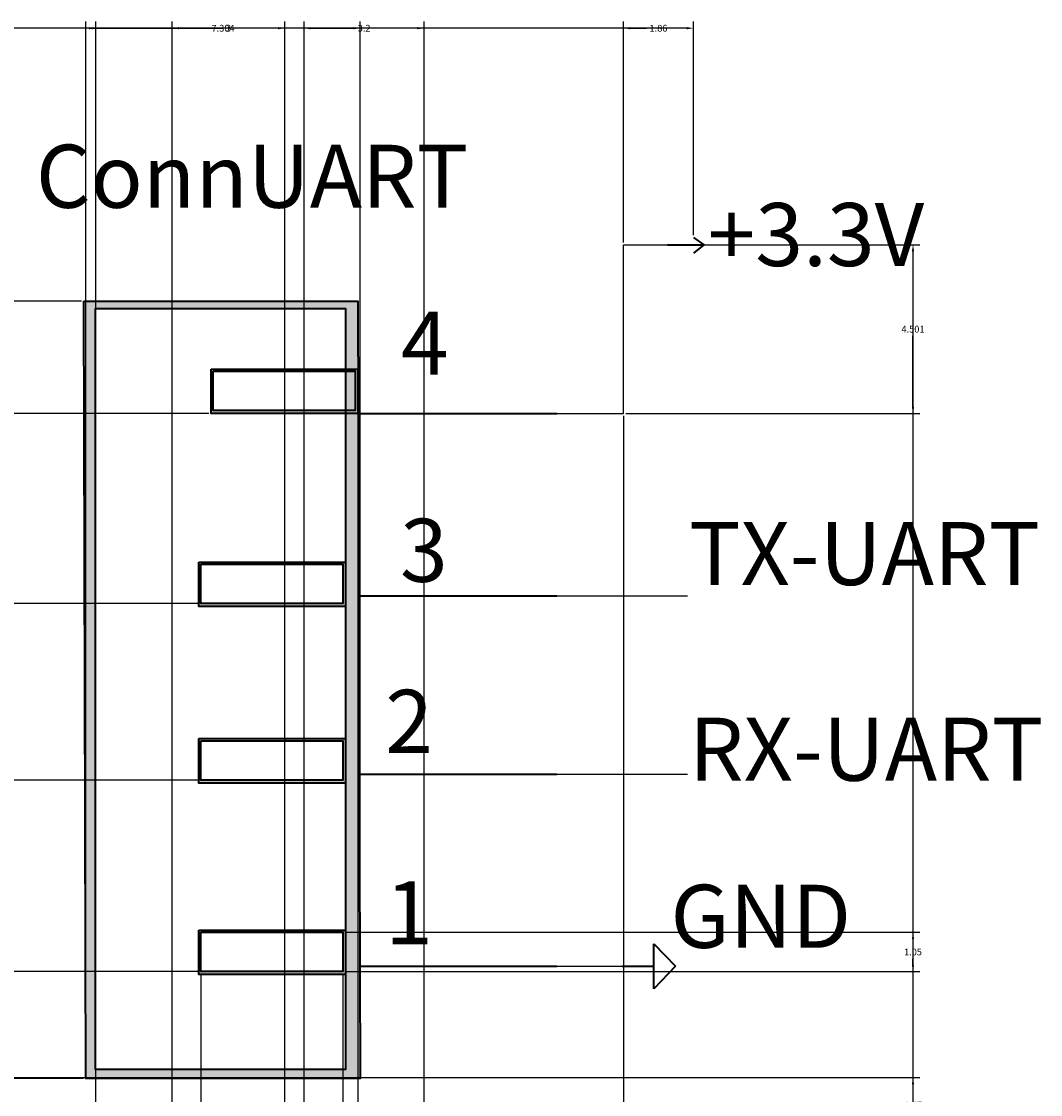
# Model space of a CAD drawing. Units: inches. Extents: x 23 to 132, y 5 to 105.
# Tile 14 of 14: x 105 to 132, y 77 to 105. Entities that reach past the tile are written whole.
import ezdxf

# ---------------------------------------------------------------- set-up
doc = ezdxf.new("R2010")
doc.units = ezdxf.units.IN
doc.header["$MEASUREMENT"] = 0
for name, color, linetype, lineweight in [('A-ANNO-DIMS', 2, 'Continuous', 18), ('E-ANNO-IDEN', 4, 'Continuous', 18), ('E-ANNO-TEXT', 3, 'Continuous', 18), ('E-SYMB', 1, 'Continuous', 35), ('E-SYMB-PATT', 1, 'Continuous', 18), ('E-WIRE', 3, 'Continuous', 25)]:
    doc.layers.add(name, color=color, linetype=linetype, lineweight=lineweight)
doc.styles.get("Standard").update_dxf_attribs({"font": 'arial.ttf'})
doc.dimstyles.get("Standard").update_dxf_attribs({"dimtxt": 0.18, "dimasz": 0.18, "dimexe": 0.18, "dimexo": 0.0625, "dimgap": 0.09, "dimtad": 0, "dimtih": 1, "dimtoh": 1, "dimdec": 4, "dimzin": 0, "dimdsep": 46, "dimtxsty": 'Standard', "dimcen": 0.09, "dimadec": 0, "dimazin": 0, "dimtfac": 1, "dimtdec": 4, "dimtofl": 0, "dimtmove": 0, "dimatfit": 3, "dimfxl": 1, "dimtolj": 1, "dimtzin": 0, "dimarcsym": 0})

# ---------------------------------------------------------------- blocks, each defined once
blk = doc.blocks.new('*D2')
at = {"layer": 'A-ANNO-DIMS', "color": 0, "lineweight": -2, "transparency": 16777216}
for p, q in [((28.697, 66.272), (28.697, 105.232)), ((123.211, 99.539), (123.211, 105.232)), ((28.877, 105.052), (75.577, 105.052)), ((123.031, 105.052), (76.33, 105.052))]:
    blk.add_line(p, q, dxfattribs=at)
at = {"layer": 'A-ANNO-DIMS', "color": 0, "transparency": 16777216}
for points in [[(28.877, 105.082), (28.877, 105.022), (28.697, 105.052)], [(123.031, 105.082), (123.031, 105.022), (123.211, 105.052)]]:
    blk.add_solid(points, dxfattribs=at)
at = {"layer": 'Defpoints', "color": 0, "transparency": 16777216}
for p in [(123.211, 105.052), (123.211, 99.477), (28.697, 66.21)]:
    blk.add_point(p, dxfattribs=at)
at = {"layer": 'A-ANNO-DIMS', "color": 0, "transparency": 16777216, "insert": (75.954, 105.052), "char_height": 0.18, "attachment_point": 5}
blk.add_mtext('\\A1;94.51', dxfattribs=at)
blk = doc.blocks.new('*D3')
at = {"layer": 'A-ANNO-DIMS', "color": 0, "lineweight": -2, "transparency": 16777216}
for p, q in [((121.409, 99.285), (129.239, 99.285)), ((129.059, 99.105), (129.059, 55.423)), ((129.059, 11.378), (129.059, 55.06)), ((72.981, 11.198), (129.239, 11.198))]:
    blk.add_line(p, q, dxfattribs=at)
at = {"layer": 'A-ANNO-DIMS', "color": 0, "transparency": 16777216}
for points in [[(129.029, 99.105), (129.089, 99.105), (129.059, 99.285)], [(129.029, 11.378), (129.089, 11.378), (129.059, 11.198)]]:
    blk.add_solid(points, dxfattribs=at)
at = {"layer": 'Defpoints', "color": 0, "transparency": 16777216}
for p in [(121.346, 99.285), (129.059, 99.285), (72.919, 11.198)]:
    blk.add_point(p, dxfattribs=at)
at = {"layer": 'A-ANNO-DIMS', "color": 0, "transparency": 16777216, "insert": (129.059, 55.241), "char_height": 0.18, "attachment_point": 5}
blk.add_mtext('\\A1;88.09', dxfattribs=at)
blk = doc.blocks.new('*D15')
at = {"layer": 'A-ANNO-DIMS', "color": 0, "lineweight": -2, "transparency": 16777216}
for p, q in [((50.327, 77.095), (129.239, 77.095)), ((129.059, 76.915), (129.059, 76.538)), ((129.059, 75.801), (129.059, 76.177)), ((47.783, 75.621), (129.239, 75.621))]:
    blk.add_line(p, q, dxfattribs=at)
at = {"layer": 'A-ANNO-DIMS', "color": 0, "transparency": 16777216}
for points in [[(129.029, 76.915), (129.089, 76.915), (129.059, 77.095)], [(129.029, 75.801), (129.089, 75.801), (129.059, 75.621)]]:
    blk.add_solid(points, dxfattribs=at)
at = {"layer": 'Defpoints', "color": 0, "transparency": 16777216}
for p in [(50.265, 77.095), (47.72, 75.621), (129.059, 75.621)]:
    blk.add_point(p, dxfattribs=at)
at = {"layer": 'A-ANNO-DIMS', "color": 0, "transparency": 16777216, "insert": (129.059, 76.358), "char_height": 0.18, "attachment_point": 5}
blk.add_mtext('\\A1;1.47', dxfattribs=at)
blk = doc.blocks.new('*D24')
at = {"layer": 'A-ANNO-DIMS', "color": 0, "lineweight": -2, "transparency": 16777216}
for p, q in [((81.032, 77.095), (129.239, 77.095)), ((129.059, 76.915), (129.059, 76.509)), ((129.059, 75.739), (129.059, 76.145)), ((83.576, 75.559), (129.239, 75.559))]:
    blk.add_line(p, q, dxfattribs=at)
at = {"layer": 'A-ANNO-DIMS', "color": 0, "transparency": 16777216}
for points in [[(129.029, 76.915), (129.089, 76.915), (129.059, 77.095)], [(129.029, 75.739), (129.089, 75.739), (129.059, 75.559)]]:
    blk.add_solid(points, dxfattribs=at)
at = {"layer": 'Defpoints', "color": 0, "transparency": 16777216}
for p in [(80.969, 77.095), (83.514, 75.559), (129.059, 75.559)]:
    blk.add_point(p, dxfattribs=at)
at = {"layer": 'A-ANNO-DIMS', "color": 0, "transparency": 16777216, "insert": (129.059, 76.327), "char_height": 0.18, "attachment_point": 5}
blk.add_mtext('\\A1;1.54', dxfattribs=at)
blk = doc.blocks.new('*D49')
at = {"layer": 'A-ANNO-DIMS', "color": 0, "lineweight": -2, "transparency": 16777216}
for p, q in [((83.514, 75.622), (83.514, 105.232)), ((107.287, 75.622), (107.287, 105.232)), ((83.694, 105.052), (94.936, 105.052)), ((107.107, 105.052), (95.865, 105.052))]:
    blk.add_line(p, q, dxfattribs=at)
at = {"layer": 'A-ANNO-DIMS', "color": 0, "transparency": 16777216}
for points in [[(83.694, 105.082), (83.694, 105.022), (83.514, 105.052)], [(107.107, 105.082), (107.107, 105.022), (107.287, 105.052)]]:
    blk.add_solid(points, dxfattribs=at)
at = {"layer": 'Defpoints', "color": 0, "transparency": 16777216}
for p in [(107.287, 105.052), (83.514, 75.559), (107.287, 75.559)]:
    blk.add_point(p, dxfattribs=at)
at = {"layer": 'A-ANNO-DIMS', "color": 0, "transparency": 16777216, "insert": (95.4, 105.052), "char_height": 0.18, "attachment_point": 5}
blk.add_mtext('\\A1;23.774', dxfattribs=at)
blk = doc.blocks.new('*D77')
at = {"layer": 'A-ANNO-DIMS', "color": 0, "lineweight": -2, "transparency": 16777216}
for p, q in [((112.835, 67.751), (112.835, 105.232)), ((116.035, 67.751), (116.035, 105.232)), ((113.015, 105.052), (114.182, 105.052)), ((115.855, 105.052), (114.688, 105.052))]:
    blk.add_line(p, q, dxfattribs=at)
at = {"layer": 'A-ANNO-DIMS', "color": 0, "transparency": 16777216}
for points in [[(113.015, 105.082), (113.015, 105.022), (112.835, 105.052)], [(115.855, 105.082), (115.855, 105.022), (116.035, 105.052)]]:
    blk.add_solid(points, dxfattribs=at)
at = {"layer": 'Defpoints', "color": 0, "transparency": 16777216}
for p in [(116.035, 105.052), (112.835, 67.688), (116.035, 67.688)]:
    blk.add_point(p, dxfattribs=at)
at = {"layer": 'A-ANNO-DIMS', "color": 0, "transparency": 16777216, "insert": (114.435, 105.052), "char_height": 0.18, "attachment_point": 5}
blk.add_mtext('\\A1;3.2', dxfattribs=at)
blk = doc.blocks.new('*D82')
at = {"layer": 'A-ANNO-DIMS', "color": 0, "lineweight": -2, "transparency": 16777216}
for p, q in [((109.322, 56.302), (109.322, 105.232)), ((112.322, 56.302), (112.322, 105.232)), ((109.502, 105.052), (110.673, 105.052)), ((112.142, 105.052), (110.971, 105.052))]:
    blk.add_line(p, q, dxfattribs=at)
at = {"layer": 'A-ANNO-DIMS', "color": 0, "transparency": 16777216}
for points in [[(109.502, 105.082), (109.502, 105.022), (109.322, 105.052)], [(112.142, 105.082), (112.142, 105.022), (112.322, 105.052)]]:
    blk.add_solid(points, dxfattribs=at)
at = {"layer": 'Defpoints', "color": 0, "transparency": 16777216}
for p in [(112.322, 105.052), (109.322, 56.24), (112.322, 56.24)]:
    blk.add_point(p, dxfattribs=at)
at = {"layer": 'A-ANNO-DIMS', "color": 0, "transparency": 16777216, "insert": (110.822, 105.052), "char_height": 0.18, "attachment_point": 5}
blk.add_mtext('\\A1;3', dxfattribs=at)
blk = doc.blocks.new('*D84')
at = {"layer": 'A-ANNO-DIMS', "color": 0, "lineweight": -2, "transparency": 16777216}
for p, q in [((107.026, 77.134), (107.026, 105.232)), ((114.33, 77.134), (114.33, 105.232)), ((107.206, 105.052), (110.285, 105.052)), ((114.15, 105.052), (111.071, 105.052))]:
    blk.add_line(p, q, dxfattribs=at)
at = {"layer": 'A-ANNO-DIMS', "color": 0, "transparency": 16777216}
for points in [[(107.206, 105.082), (107.206, 105.022), (107.026, 105.052)], [(114.15, 105.082), (114.15, 105.022), (114.33, 105.052)]]:
    blk.add_solid(points, dxfattribs=at)
at = {"layer": 'Defpoints', "color": 0, "transparency": 16777216}
for p in [(114.33, 105.052), (107.026, 77.071), (114.33, 77.071)]:
    blk.add_point(p, dxfattribs=at)
at = {"layer": 'A-ANNO-DIMS', "color": 0, "transparency": 16777216, "insert": (110.678, 105.052), "char_height": 0.18, "attachment_point": 5}
blk.add_mtext('\\A1;7.304', dxfattribs=at)
blk = doc.blocks.new('*D85')
at = {"layer": 'A-ANNO-DIMS', "color": 0, "lineweight": -2, "transparency": 16777216}
for p, q in [((106.903, 97.776), (22.942, 97.776)), ((23.122, 97.596), (23.122, 87.606)), ((23.122, 77.251), (23.122, 87.242)), ((106.964, 77.071), (22.942, 77.071))]:
    blk.add_line(p, q, dxfattribs=at)
at = {"layer": 'A-ANNO-DIMS', "color": 0, "transparency": 16777216}
for points in [[(23.092, 97.596), (23.152, 97.596), (23.122, 97.776)], [(23.092, 77.251), (23.152, 77.251), (23.122, 77.071)]]:
    blk.add_solid(points, dxfattribs=at)
at = {"layer": 'Defpoints', "color": 0, "transparency": 16777216}
for p in [(23.122, 97.776), (106.965, 97.776), (107.026, 77.071)]:
    blk.add_point(p, dxfattribs=at)
at = {"layer": 'A-ANNO-DIMS', "color": 0, "transparency": 16777216, "insert": (23.122, 87.424), "char_height": 0.18, "attachment_point": 5}
blk.add_mtext('\\A1;20.705', dxfattribs=at)
blk = doc.blocks.new('*D86')
at = {"layer": 'A-ANNO-DIMS', "color": 0, "lineweight": -2, "transparency": 16777216}
for p, q in [((110.027, 79.916), (22.942, 79.916)), ((23.122, 79.736), (23.122, 78.675)), ((23.122, 77.251), (23.122, 78.312)), ((106.964, 77.071), (22.942, 77.071))]:
    blk.add_line(p, q, dxfattribs=at)
at = {"layer": 'A-ANNO-DIMS', "color": 0, "transparency": 16777216}
for points in [[(23.092, 79.736), (23.152, 79.736), (23.122, 79.916)], [(23.092, 77.251), (23.152, 77.251), (23.122, 77.071)]]:
    blk.add_solid(points, dxfattribs=at)
at = {"layer": 'Defpoints', "color": 0, "transparency": 16777216}
for p in [(23.122, 79.916), (110.089, 79.916), (107.026, 77.071)]:
    blk.add_point(p, dxfattribs=at)
at = {"layer": 'A-ANNO-DIMS', "color": 0, "transparency": 16777216, "insert": (23.122, 78.493), "char_height": 0.18, "attachment_point": 5}
blk.add_mtext('\\A1;2.84', dxfattribs=at)
blk = doc.blocks.new('*D87')
at = {"layer": 'A-ANNO-DIMS', "color": 0, "lineweight": -2, "transparency": 16777216}
for p, q in [((110.027, 85.021), (22.942, 85.021)), ((23.122, 84.841), (23.122, 82.65)), ((23.122, 80.096), (23.122, 82.286)), ((110.027, 79.916), (22.942, 79.916))]:
    blk.add_line(p, q, dxfattribs=at)
at = {"layer": 'A-ANNO-DIMS', "color": 0, "transparency": 16777216}
for points in [[(23.092, 84.841), (23.152, 84.841), (23.122, 85.021)], [(23.092, 80.096), (23.152, 80.096), (23.122, 79.916)]]:
    blk.add_solid(points, dxfattribs=at)
at = {"layer": 'Defpoints', "color": 0, "transparency": 16777216}
for p in [(23.122, 85.021), (110.089, 85.021), (110.089, 79.916)]:
    blk.add_point(p, dxfattribs=at)
at = {"layer": 'A-ANNO-DIMS', "color": 0, "transparency": 16777216, "insert": (23.122, 82.468), "char_height": 0.18, "attachment_point": 5}
blk.add_mtext('\\A1;5.105', dxfattribs=at)
blk = doc.blocks.new('*D88')
at = {"layer": 'A-ANNO-DIMS', "color": 0, "lineweight": -2, "transparency": 16777216}
for p, q in [((110.027, 89.722), (22.942, 89.722)), ((23.122, 89.542), (23.122, 87.554)), ((23.122, 85.201), (23.122, 87.19)), ((110.027, 85.021), (22.942, 85.021))]:
    blk.add_line(p, q, dxfattribs=at)
at = {"layer": 'A-ANNO-DIMS', "color": 0, "transparency": 16777216}
for points in [[(23.092, 89.542), (23.152, 89.542), (23.122, 89.722)], [(23.092, 85.201), (23.152, 85.201), (23.122, 85.021)]]:
    blk.add_solid(points, dxfattribs=at)
at = {"layer": 'Defpoints', "color": 0, "transparency": 16777216}
for p in [(23.122, 89.722), (110.089, 89.722), (110.089, 85.021)]:
    blk.add_point(p, dxfattribs=at)
at = {"layer": 'A-ANNO-DIMS', "color": 0, "transparency": 16777216, "insert": (23.122, 87.372), "char_height": 0.18, "attachment_point": 5}
blk.add_mtext('\\A1;4.702', dxfattribs=at)
blk = doc.blocks.new('*D89')
at = {"layer": 'A-ANNO-DIMS', "color": 0, "lineweight": -2, "transparency": 16777216}
for p, q in [((110.298, 94.783), (22.942, 94.783)), ((23.122, 94.603), (23.122, 92.435)), ((23.122, 89.902), (23.122, 92.071)), ((110.027, 89.722), (22.942, 89.722))]:
    blk.add_line(p, q, dxfattribs=at)
at = {"layer": 'A-ANNO-DIMS', "color": 0, "transparency": 16777216}
for points in [[(23.092, 94.603), (23.152, 94.603), (23.122, 94.783)], [(23.092, 89.902), (23.152, 89.902), (23.122, 89.722)]]:
    blk.add_solid(points, dxfattribs=at)
at = {"layer": 'Defpoints', "color": 0, "transparency": 16777216}
for p in [(23.122, 94.783), (110.36, 94.783), (110.089, 89.722)]:
    blk.add_point(p, dxfattribs=at)
at = {"layer": 'A-ANNO-DIMS', "color": 0, "transparency": 16777216, "insert": (23.122, 92.253), "char_height": 0.18, "attachment_point": 5}
blk.add_mtext('\\A1;5.061', dxfattribs=at)
blk = doc.blocks.new('*D90')
at = {"layer": 'A-ANNO-DIMS', "color": 0, "lineweight": -2, "transparency": 16777216}
for p, q in [((106.903, 97.776), (22.942, 97.776)), ((23.122, 97.596), (23.122, 96.462)), ((23.122, 94.963), (23.122, 96.098)), ((110.298, 94.783), (22.942, 94.783))]:
    blk.add_line(p, q, dxfattribs=at)
at = {"layer": 'A-ANNO-DIMS', "color": 0, "transparency": 16777216}
for points in [[(23.092, 97.596), (23.152, 97.596), (23.122, 97.776)], [(23.092, 94.963), (23.152, 94.963), (23.122, 94.783)]]:
    blk.add_solid(points, dxfattribs=at)
at = {"layer": 'Defpoints', "color": 0, "transparency": 16777216}
for p in [(23.122, 97.776), (106.965, 97.776), (110.36, 94.783)]:
    blk.add_point(p, dxfattribs=at)
at = {"layer": 'A-ANNO-DIMS', "color": 0, "transparency": 16777216, "insert": (23.122, 96.28), "char_height": 0.18, "attachment_point": 5}
blk.add_mtext('\\A1;2.993', dxfattribs=at)
blk = doc.blocks.new('*D91')
at = {"layer": 'A-ANNO-DIMS', "color": 0, "lineweight": -2, "transparency": 16777216}
for p, q in [((110.089, 79.853), (110.089, 5.443)), ((113.872, 79.853), (113.872, 5.443)), ((110.269, 5.623), (111.587, 5.623)), ((113.692, 5.623), (112.374, 5.623))]:
    blk.add_line(p, q, dxfattribs=at)
at = {"layer": 'A-ANNO-DIMS', "color": 0, "transparency": 16777216}
for points in [[(110.269, 5.653), (110.269, 5.593), (110.089, 5.623)], [(113.692, 5.653), (113.692, 5.593), (113.872, 5.623)]]:
    blk.add_solid(points, dxfattribs=at)
at = {"layer": 'Defpoints', "color": 0, "transparency": 16777216}
for p in [(110.089, 79.916), (113.872, 79.916), (113.872, 5.623)]:
    blk.add_point(p, dxfattribs=at)
at = {"layer": 'A-ANNO-DIMS', "color": 0, "transparency": 16777216, "insert": (111.981, 5.623), "char_height": 0.18, "attachment_point": 5}
blk.add_mtext('\\A1;3.783', dxfattribs=at)
blk = doc.blocks.new('*D92')
at = {"layer": 'A-ANNO-DIMS', "color": 0, "lineweight": -2, "transparency": 16777216}
for p, q in [((113.934, 80.964), (129.239, 80.964)), ((129.059, 80.784), (129.059, 80.622)), ((129.059, 80.096), (129.059, 80.258)), ((113.934, 79.916), (129.239, 79.916))]:
    blk.add_line(p, q, dxfattribs=at)
at = {"layer": 'A-ANNO-DIMS', "color": 0, "transparency": 16777216}
for points in [[(129.029, 80.784), (129.089, 80.784), (129.059, 80.964)], [(129.029, 80.096), (129.089, 80.096), (129.059, 79.916)]]:
    blk.add_solid(points, dxfattribs=at)
at = {"layer": 'Defpoints', "color": 0, "transparency": 16777216}
for p in [(113.872, 80.964), (129.059, 80.964), (113.872, 79.916)]:
    blk.add_point(p, dxfattribs=at)
at = {"layer": 'A-ANNO-DIMS', "color": 0, "transparency": 16777216, "insert": (129.059, 80.44), "char_height": 0.18, "attachment_point": 5}
blk.add_mtext('\\A1;1.05', dxfattribs=at)
blk = doc.blocks.new('*D93')
at = {"layer": 'A-ANNO-DIMS', "color": 0, "lineweight": -2, "transparency": 16777216}
for p, q in [((114.269, 94.721), (114.269, 5.443)), ((121.346, 94.721), (121.346, 5.443)), ((114.449, 5.623), (117.415, 5.623)), ((121.166, 5.623), (118.201, 5.623))]:
    blk.add_line(p, q, dxfattribs=at)
at = {"layer": 'A-ANNO-DIMS', "color": 0, "transparency": 16777216}
for points in [[(114.449, 5.653), (114.449, 5.593), (114.269, 5.623)], [(121.166, 5.653), (121.166, 5.593), (121.346, 5.623)]]:
    blk.add_solid(points, dxfattribs=at)
at = {"layer": 'Defpoints', "color": 0, "transparency": 16777216}
for p in [(114.269, 94.783), (121.346, 94.783), (121.346, 5.623)]:
    blk.add_point(p, dxfattribs=at)
at = {"layer": 'A-ANNO-DIMS', "color": 0, "transparency": 16777216, "insert": (117.808, 5.623), "char_height": 0.18, "attachment_point": 5}
blk.add_mtext('\\A1;7.077', dxfattribs=at)
blk = doc.blocks.new('*D94')
at = {"layer": 'A-ANNO-DIMS', "color": 0, "lineweight": -2, "transparency": 16777216}
for p, q in [((121.409, 99.285), (129.239, 99.285)), ((129.059, 99.105), (129.059, 97.216)), ((129.059, 94.963), (129.059, 96.852)), ((121.409, 94.783), (129.239, 94.783))]:
    blk.add_line(p, q, dxfattribs=at)
at = {"layer": 'A-ANNO-DIMS', "color": 0, "transparency": 16777216}
for points in [[(129.029, 99.105), (129.089, 99.105), (129.059, 99.285)], [(129.029, 94.963), (129.089, 94.963), (129.059, 94.783)]]:
    blk.add_solid(points, dxfattribs=at)
at = {"layer": 'Defpoints', "color": 0, "transparency": 16777216}
for p in [(121.346, 99.285), (129.059, 99.285), (121.346, 94.783)]:
    blk.add_point(p, dxfattribs=at)
at = {"layer": 'A-ANNO-DIMS', "color": 0, "transparency": 16777216, "insert": (129.059, 97.034), "char_height": 0.18, "attachment_point": 5}
blk.add_mtext('\\A1;4.501', dxfattribs=at)
blk = doc.blocks.new('*D95')
at = {"layer": 'A-ANNO-DIMS', "color": 0, "lineweight": -2, "transparency": 16777216}
for p, q in [((121.346, 99.347), (121.346, 105.232)), ((123.211, 99.539), (123.211, 105.232)), ((121.526, 105.052), (121.963, 105.052)), ((123.031, 105.052), (122.594, 105.052))]:
    blk.add_line(p, q, dxfattribs=at)
at = {"layer": 'A-ANNO-DIMS', "color": 0, "transparency": 16777216}
for points in [[(121.526, 105.082), (121.526, 105.022), (121.346, 105.052)], [(123.031, 105.082), (123.031, 105.022), (123.211, 105.052)]]:
    blk.add_solid(points, dxfattribs=at)
at = {"layer": 'Defpoints', "color": 0, "transparency": 16777216}
for p in [(123.211, 105.052), (121.346, 99.285), (123.211, 99.477)]:
    blk.add_point(p, dxfattribs=at)
at = {"layer": 'A-ANNO-DIMS', "color": 0, "transparency": 16777216, "insert": (122.278, 105.052), "char_height": 0.18, "attachment_point": 5}
blk.add_mtext('\\A1;1.86', dxfattribs=at)

msp = doc.modelspace()

# ---------------------------------------------------------------- hatches: boundary and pattern name
at = {"layer": 'E-SYMB-PATT'}
h = msp.add_hatch(color=256, dxfattribs=at)
h.dxf.hatch_style = 1
h.paths.add_polyline_path([(107.026, 77.0711), (114.3301, 77.0711), (114.2693, 97.7764), (106.9652, 97.7764)])
h.paths.add_polyline_path([(113.9442, 77.3093), (107.2756, 77.3093), (107.2756, 97.5825), (113.9442, 97.5825)], flags=16)
h = msp.add_hatch(color=256, dxfattribs=at)
h.dxf.hatch_style = 1
h.paths.add_polyline_path([(110.36, 94.7833), (114.2693, 94.7833), (114.2693, 95.9665), (110.36, 95.9665)])
h.paths.add_polyline_path([(110.4142, 94.8634), (114.1969, 94.8634), (114.1969, 95.9116), (110.4142, 95.9116)], flags=16)
h = msp.add_hatch(color=256, dxfattribs=at)
h.dxf.hatch_style = 1
h.paths.add_polyline_path([(110.035, 89.6423), (113.9442, 89.6423), (113.9442, 90.8256), (110.035, 90.8256)])
h.paths.add_polyline_path([(110.0892, 89.7224), (113.8719, 89.7224), (113.8719, 90.7706), (110.0892, 90.7706)], flags=16)
h = msp.add_hatch(color=256, dxfattribs=at)
h.dxf.hatch_style = 1
h.paths.add_polyline_path([(110.035, 84.9408), (113.9442, 84.9408), (113.9442, 86.124), (110.035, 86.124)])
h.paths.add_polyline_path([(110.0892, 85.0209), (113.8719, 85.0209), (113.8719, 86.0691), (110.0892, 86.0691)], flags=16)
h = msp.add_hatch(color=256, dxfattribs=at)
h.dxf.hatch_style = 1
h.paths.add_polyline_path([(110.035, 79.8357), (113.9442, 79.8357), (113.9442, 81.0189), (110.035, 81.0189)])
h.paths.add_polyline_path([(110.0892, 79.9158), (113.8719, 79.9158), (113.8719, 80.964), (110.0892, 80.964)], flags=16)

# ---------------------------------------------------------------- linework, layer by layer
at = {"layer": 'E-SYMB'}
for p, q in [((122.5212, 99.2846), (123.4839, 99.2846)), ((123.2107, 99.477), (123.4839, 99.2846)), ((123.4839, 99.2846), (123.2107, 99.0613)), ((114.2693, 94.7833), (119.5739, 94.7833)), ((114.2923, 89.9272), (119.5739, 89.9272)), ((114.3063, 85.1757), (119.5739, 85.1757)), ((122.1572, 80.0664), (122.1572, 80.6565)), ((122.1572, 80.6565), (122.7316, 80.0664)), ((114.3213, 80.0664), (119.5739, 80.0664)), ((121.3114, 80.0664), (122.1572, 80.0664)), ((122.7316, 80.0664), (122.1572, 79.4607)), ((122.1572, 79.4607), (122.1572, 80.0664))]:
    msp.add_line(p, q, dxfattribs=at)
for points in [[(106.9652, 97.7764), (114.2693, 97.7764), (114.3301, 77.0711), (107.026, 77.0711)], [(107.2756, 97.5825), (113.9442, 97.5825), (113.9442, 77.3093), (107.2756, 77.3093)], [(110.36, 95.9665), (114.2693, 95.9665), (114.2693, 94.7833), (110.36, 94.7833)], [(110.4142, 95.9116), (114.1969, 95.9116), (114.1969, 94.8634), (110.4142, 94.8634)], [(110.035, 90.8256), (113.9442, 90.8256), (113.9442, 89.6423), (110.035, 89.6423)], [(110.0892, 90.7706), (113.8719, 90.7706), (113.8719, 89.7224), (110.0892, 89.7224)], [(110.035, 86.124), (113.9442, 86.124), (113.9442, 84.9408), (110.035, 84.9408)], [(110.0892, 86.0691), (113.8719, 86.0691), (113.8719, 85.0209), (110.0892, 85.0209)], [(110.035, 81.0189), (113.9442, 81.0189), (113.9442, 79.8357), (110.035, 79.8357)], [(110.0892, 80.964), (113.8719, 80.964), (113.8719, 79.9158), (110.0892, 79.9158)]]:
    msp.add_lwpolyline(points, close=True, dxfattribs=at)
at = {"layer": 'E-WIRE'}
for p, q in [((121.3461, 94.7833), (121.3461, 99.2846)), ((121.3461, 99.2846), (122.5212, 99.2846)), ((119.5739, 94.7833), (121.3461, 94.7833)), ((119.5739, 89.9272), (123.0523, 89.9272)), ((119.5739, 85.1757), (123.0523, 85.1757)), ((119.5739, 80.0664), (121.3114, 80.0664))]:
    msp.add_line(p, q, dxfattribs=at)

# ---------------------------------------------------------------- texts
at = {"layer": 'E-ANNO-IDEN'}
for s, p in [('ConnUART', (105.6909, 100.268)), ('+3.3V', (123.5872, 98.715)), ('TX-UART', (123.0931, 90.216)), ('RX-UART', (123.0931, 85.0026)), ('GND', (122.5981, 80.5507))]:
    msp.add_text(s, height=1.67943, dxfattribs=at).set_placement(p)
at = {"layer": 'E-ANNO-TEXT'}
for s, p in [('4', (115.4171, 95.8223)), ('3', (115.393, 90.3025)), ('2', (114.997, 85.745)), ('1', (114.9967, 80.645))]:
    msp.add_text(s, height=1.6794, dxfattribs=at).set_placement(p)

# ---------------------------------------------------------------- dimensions: what is measured, and where the dimension line sits
at = {"layer": 'A-ANNO-DIMS'}
for base, p1, p2, override, picture, middle in [((123.2107, 105.052), (28.6965, 66.2099), (123.2107, 99.477), {"dimdec": 2, "dimlfac": 1, "dimrnd": 0, "dimzin": 0, "dimdsep": 46, "dimlunit": 2}, '*D2', (75.9536, 105.052)), ((107.2874, 105.052), (83.5136, 75.5594), (107.2874, 75.5594), {"dimdec": 3, "dimlfac": 1, "dimrnd": 0, "dimzin": 0, "dimdsep": 46, "dimlunit": 2}, '*D49', (95.4005, 105.052)), ((114.3301, 105.052), (107.026, 77.0711), (114.3301, 77.0711), {"dimdec": 3, "dimlfac": 1, "dimrnd": 0, "dimzin": 0, "dimdsep": 46, "dimlunit": 2}, '*D84', (110.6781, 105.052)), ((112.3219, 105.052), (109.3219, 56.2399), (112.3219, 56.2399), {"dimdec": 0, "dimlfac": 1, "dimrnd": 0, "dimzin": 0, "dimdsep": 46, "dimlunit": 2}, '*D82', (110.8219, 105.052)), ((116.0352, 105.052), (112.8351, 67.6881), (116.0352, 67.6881), {"dimdec": 1, "dimlfac": 1, "dimrnd": 0, "dimzin": 0, "dimdsep": 46, "dimlunit": 2}, '*D77', (114.4351, 105.052)), ((123.2107, 105.052), (121.3461, 99.2846), (123.2107, 99.477), {"dimdec": 2, "dimlfac": 1, "dimrnd": 0, "dimzin": 0, "dimdsep": 46, "dimlunit": 2}, '*D95', (122.2784, 105.052)), ((121.3461, 5.6233), (114.2693, 94.7833), (121.3461, 94.7833), {"dimdec": 3, "dimlfac": 1, "dimrnd": 0, "dimzin": 0, "dimdsep": 46, "dimlunit": 2}, '*D93', (117.8077, 5.6233)), ((113.8719, 5.6233), (110.0892, 79.9158), (113.8719, 79.9158), {"dimdec": 3, "dimlfac": 1, "dimrnd": 0, "dimzin": 0, "dimdsep": 46, "dimlunit": 2}, '*D91', (111.9805, 5.6233))]:
    dim = msp.add_linear_dim(base=base, p1=p1, p2=p2, dimstyle='Standard', override=override, dxfattribs=at)
    dim.commit()
    dim.dimension.update_dxf_attribs({"geometry": picture, "text_midpoint": middle})
for base, p1, p2, override, picture, middle in [((129.0589, 99.2846), (72.9188, 11.1983), (121.3461, 99.2846), {"dimdec": 2, "dimlfac": 1, "dimrnd": 0, "dimzin": 0, "dimdsep": 46, "dimlunit": 2}, '*D3', (129.0589, 55.2415)), ((129.0589, 99.2846), (121.3461, 94.7833), (121.3461, 99.2846), {"dimdec": 3, "dimlfac": 1, "dimrnd": 0, "dimzin": 0, "dimdsep": 46, "dimlunit": 2}, '*D94', (129.0589, 97.034)), ((23.1215, 97.7764), (107.026, 77.0711), (106.9652, 97.7764), {"dimdec": 3, "dimlfac": 1, "dimrnd": 0, "dimzin": 0, "dimdsep": 46, "dimlunit": 2}, '*D85', (23.1215, 87.4238)), ((23.1215, 97.7764), (110.36, 94.7833), (106.9652, 97.7764), {"dimdec": 3, "dimlfac": 1, "dimrnd": 0, "dimzin": 0, "dimdsep": 46, "dimlunit": 2}, '*D90', (23.1215, 96.2798)), ((23.1215, 94.7833), (110.0892, 89.7224), (110.36, 94.7833), {"dimdec": 3, "dimlfac": 1, "dimrnd": 0, "dimzin": 0, "dimdsep": 46, "dimlunit": 2}, '*D89', (23.1215, 92.2528)), ((23.12152, 89.7224), (110.08916, 85.02085), (110.08916, 89.7224), {"dimdec": 3, "dimlfac": 1, "dimrnd": 0, "dimzin": 0, "dimdsep": 46, "dimlunit": 2}, '*D88', (23.12152, 87.37162)), ((23.1215, 85.0209), (110.0892, 79.9158), (110.0892, 85.0209), {"dimdec": 3, "dimlfac": 1, "dimrnd": 0, "dimzin": 0, "dimdsep": 46, "dimlunit": 2}, '*D87', (23.1215, 82.4683)), ((129.0589, 80.964), (113.8719, 79.9158), (113.8719, 80.964), {"dimdec": 2, "dimlfac": 1, "dimrnd": 0, "dimzin": 0, "dimdsep": 46, "dimlunit": 2}, '*D92', (129.0589, 80.4399)), ((23.1215, 79.9158), (107.026, 77.0711), (110.0892, 79.9158), {"dimdec": 2, "dimlfac": 1, "dimrnd": 0, "dimzin": 0, "dimdsep": 46, "dimlunit": 2}, '*D86', (23.1215, 78.4935)), ((129.0589, 75.6207), (50.2646, 77.095), (47.7202, 75.6207), {"dimdec": 2, "dimlfac": 1, "dimrnd": 0, "dimzin": 0, "dimdsep": 46, "dimlunit": 2}, '*D15', (129.0589, 76.3579)), ((129.0589, 75.5594), (80.9692, 77.095), (83.5136, 75.5594), {"dimdec": 2, "dimlfac": 1, "dimrnd": 0, "dimzin": 0, "dimdsep": 46, "dimlunit": 2}, '*D24', (129.0589, 76.3272))]:
    dim = msp.add_linear_dim(base=base, p1=p1, p2=p2, angle=90, dimstyle='Standard', override=override, dxfattribs=at)
    dim.commit()
    dim.dimension.update_dxf_attribs({"geometry": picture, "text_midpoint": middle})

doc.saveas('drawing.dxf')
